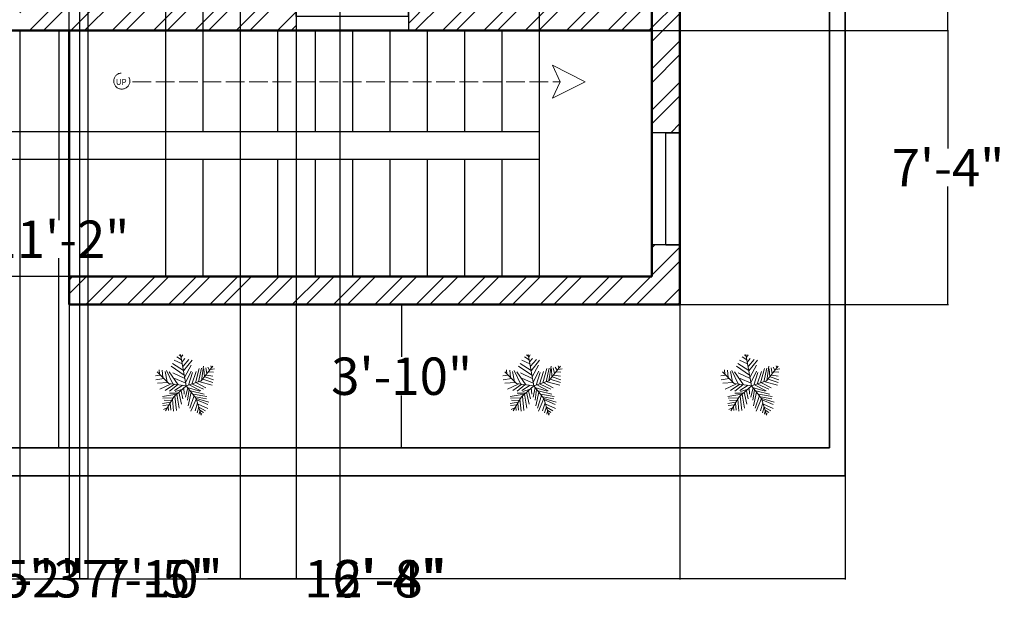
# Model space of a CAD drawing. Units: inches. Extents: x -40 to 578, y -482 to 237.
# Tile 2 of 7: x 219 to 535, y -482 to -295. Entities that reach past the tile are written whole.
import ezdxf

# ---------------------------------------------------------------- set-up
doc = ezdxf.new("R2010")
doc.units = ezdxf.units.IN
doc.header["$MEASUREMENT"] = 0
doc.linetypes.add('ACAD_ISO02W100', pattern=[15, 12, -3])
for name, color, linetype, lineweight in [('A-ANNO-DIMS', 2, 'Continuous', 18), ('A-ANNO-SYMB', 210, 'ACAD_ISO02W100', 18), ('A-FLOR-STRS', 210, 'Continuous', 25), ('A-WALL-PATT', 252, 'Continuous', 13), ('C-PROP', 3, 'Continuous', 35), ('L-PLNT', 94, 'Continuous', 13), ('WALLS', 3, 'Continuous', 50), ('WINDOWS', 241, 'Continuous', 25)]:
    doc.layers.add(name, color=color, linetype=linetype, lineweight=lineweight)
doc.styles.get("Standard").update_dxf_attribs({"font": 'arial.ttf'})
doc.dimstyles.get("Standard").update_dxf_attribs({"dimtxt": 12, "dimasz": 0.18, "dimexe": 0.18, "dimexo": 0.0625, "dimgap": 0.09, "dimtad": 0, "dimtih": 1, "dimtoh": 1, "dimdec": 0, "dimzin": 0, "dimdsep": 46, "dimlunit": 3, "dimtxsty": 'Standard', "dimcen": 0.09, "dimadec": 0, "dimazin": 0, "dimtfac": 1, "dimtdec": 0, "dimtofl": 0, "dimtmove": 0, "dimatfit": 3, "dimfxl": 1, "dimtolj": 1, "dimtzin": 0, "dimarcsym": 0})

# ---------------------------------------------------------------- blocks, each defined once
blk = doc.blocks.new('*U14')
for p, q in [((-258.7244, 1362.456), (-332.3336, 1421.4348)), ((0, 0), (-266.7, 1447.8)), ((-231.1146, 1315.2628), (-166.7002, 1421.4348)), ((-129.8956, 713.6638), (-626.7704, 1032.1544)), ((-185.1152, 1008.5578), (-553.1612, 1185.4942)), ((-221.9198, 1197.3052), (-433.5526, 1338.8594)), ((-194.31, 1102.9442), (-65.4812, 1256.284)), ((-148.3106, 914.1968), (118.5418, 1220.9018)), ((-129.8956, 701.8528), (265.7602, 1185.4942)), ((-74.7014, 418.7444), (219.7608, 961.39)), ((685.8, 228.6), (1219.2, 914.4)), ((689.0258, 230.0224), (790.2448, 914.1968)), ((1121.4862, 925.9824), (1149.0706, 831.6214)), ((-1206.4492, 501.3198), (-1418.082, 465.9376)), ((-800.1, 114.3), (-1333.5, 647.7)), ((-1234.059, 536.7274), (-1252.4486, 737.2604)), ((-1105.2302, 725.4494), (-1077.6458, 395.1732)), ((-976.4268, 666.4706), (-884.4026, 194.6402)), ((-902.8176, 713.6638), (-617.5756, 100.2538)), ((-369.1382, 53.086), (-783.1836, 642.874)), ((-93.091, 489.5342), (-700.3796, 902.3858)), ((-617.5756, 607.4918), (-74.7014, 347.98)), ((-28.6766, 171.0436), (228.9556, 678.2816)), ((100.1268, 41.275), (284.1498, 619.2774)), ((256.5654, 88.4682), (449.7832, 666.4706)), ((412.9786, 147.447), (587.8068, 796.2392)), ((560.197, 182.8292), (698.2206, 819.8358)), ((808.6344, 784.4282), (827.0494, 418.7444)), ((891.4384, 831.6214), (946.658, 572.1096)), ((919.0482, 501.3198), (1222.6798, 454.152)), ((983.4626, 867.0036), (1066.2666, 725.4494)), ((1029.462, 654.685), (1241.0948, 631.0884)), ((1112.2914, 760.8316), (1296.3144, 784.4282)), ((-1031.621, 347.98), (-1399.667, 277.1902)), ((-847.598, 159.2326), (-1326.0578, 135.636)), ((-718.7946, 88.4682), (-1215.644, -147.447)), ((-543.9664, 76.6572), (-967.2066, -206.4512)), ((0, 0), (-800.1, 114.3)), ((-405.9428, 53.086), (-764.794, -241.8334)), ((0, 0), (-571.5, -495.3)), ((-166.7002, 29.4894), (-543.9664, -206.4512)), ((-525.5514, 347.98), (-28.6766, 123.8504)), ((0, 0), (685.8, 228.6)), ((0, 0), (457.2, -571.5)), ((164.5412, 41.275), (661.416, -218.2368)), ((284.1498, 88.4682), (781.0246, -147.447)), ((458.978, 147.447), (891.4384, -88.4682)), ((615.4166, 194.6402), (1185.8752, 41.275)), ((753.4148, 312.5978), (1222.6798, 159.2326)), ((845.439, 418.7444), (1241.0948, 277.1902)), ((-442.7474, -383.3876), (-1086.8406, -477.7486)), ((-387.5278, -324.4088), (-764.794, -324.4088)), ((-166.7002, -147.447), (-507.1618, -253.619)), ((-433.5526, -383.3876), (-323.1134, -1020.3688)), ((-341.5284, -289.0012), (-221.9198, -831.6214)), ((-240.3094, -218.2368), (-157.5054, -595.7062)), ((-120.7008, -88.4682), (-93.091, -371.5766)), ((63.3222, -76.6826), (-37.8714, -513.1308)), ((44.9326, -64.897), (615.4166, -241.8334)), ((127.7366, -159.258), (54.1274, -654.685)), ((228.9556, -289.0012), (90.932, -914.1968)), ((357.759, -430.5554), (164.5412, -1020.3688)), ((192.151, -230.0224), (817.8292, -371.5766)), ((311.7596, -383.3876), (937.4378, -477.7486)), ((-718.7946, -737.2604), (-1086.8406, -796.2392)), ((-617.5756, -548.5384), (-1077.6458, -560.324)), ((-783.1836, -867.029), (-1077.6458, -902.4112)), ((-681.9646, -666.496), (-1022.4262, -654.685)), ((-571.5, -495.3), (-952.5, -1143)), ((-737.1842, -784.4536), (-709.5744, -1114.7298)), ((-635.9652, -607.5172), (-580.771, -1150.1374)), ((-525.5514, -465.963), (-451.9422, -1126.5408)), ((458.978, -572.1096), (210.5406, -1161.923)), ((514.1976, -772.6426), (403.7838, -1138.3264)), ((412.9786, -501.3452), (919.0482, -583.9206)), ((457.2, -571.5), (685.8, -1333.5)), ((468.1982, -572.1096), (1029.462, -737.2604)), ((486.5878, -642.8994), (983.4626, -843.4324)), ((541.8074, -831.6214), (992.6574, -1032.1544)), ((-875.2078, -1008.5832), (-1040.8412, -1079.3476)), ((-829.2084, -937.7934), (-810.7934, -1126.5408)), ((578.612, -961.39), (495.7826, -1232.7128)), ((578.612, -973.1756), (873.0488, -1138.3264)), ((624.6114, -1161.923), (587.8068, -1291.6916)), ((624.6114, -1102.9442), (781.0246, -1209.1162)), ((679.8056, -1268.095), (716.6102, -1291.6916))]:
    blk.add_line(p, q)
blk = doc.blocks.new('*D17')
at = {"layer": 'A-ANNO-DIMS', "color": 0, "lineweight": -2, "transparency": 16777216}
for p, q in [((229.86, -298.55), (231.51, -298.55)), ((231.33, -298.73), (231.33, -359.44)), ((231.33, -432.37), (231.33, -371.67)), ((229.86, -432.55), (231.51, -432.55))]:
    blk.add_line(p, q, dxfattribs=at)
at = {"layer": 'A-ANNO-DIMS', "color": 0, "transparency": 16777216}
for points in [[(231.3, -298.73), (231.36, -298.73), (231.33, -298.55)], [(231.3, -432.37), (231.36, -432.37), (231.33, -432.55)]]:
    blk.add_solid(points, dxfattribs=at)
at = {"layer": 'Defpoints', "color": 0, "transparency": 16777216}
for p in [(229.79, -298.55), (229.79, -432.55), (231.33, -432.55)]:
    blk.add_point(p, dxfattribs=at)
at = {"layer": 'A-ANNO-DIMS', "color": 0, "transparency": 16777216, "insert": (231.33, -365.55), "char_height": 12, "attachment_point": 5}
blk.add_mtext('\\A1;11\'-2"', dxfattribs=at)
blk = doc.blocks.new('*D18')
at = {"layer": 'A-ANNO-DIMS', "color": 0, "lineweight": -2, "transparency": 16777216}
for p, q in [((354.59, -386.55), (341.19, -386.55)), ((341.37, -386.73), (341.37, -403.33)), ((341.37, -432.37), (341.37, -415.77)), ((354.59, -432.55), (341.19, -432.55))]:
    blk.add_line(p, q, dxfattribs=at)
at = {"layer": 'A-ANNO-DIMS', "color": 0, "transparency": 16777216}
for points in [[(341.34, -386.73), (341.4, -386.73), (341.37, -386.55)], [(341.34, -432.37), (341.4, -432.37), (341.37, -432.55)]]:
    blk.add_solid(points, dxfattribs=at)
at = {"layer": 'Defpoints', "color": 0, "transparency": 16777216}
for p in [(354.65, -386.55), (341.37, -432.55), (354.65, -432.55)]:
    blk.add_point(p, dxfattribs=at)
at = {"layer": 'A-ANNO-DIMS', "color": 0, "transparency": 16777216, "insert": (341.37, -409.55), "char_height": 12, "attachment_point": 5}
blk.add_mtext('\\A1;3\'-10"', dxfattribs=at)
blk = doc.blocks.new('WIN-36IN')
for p, q in [((9, 36), (0, 36)), ((4.5, 0), (4.5, 36)), ((4.5, 36), (9, 36)), ((9, 0), (0, 0)), ((4.5, 0), (9, 0))]:
    blk.add_line(p, q)
blk = doc.blocks.new('*D38')
at = {"layer": 'A-ANNO-DIMS', "color": 0, "lineweight": -2, "transparency": 16777216}
for p, q in [((266.02, -266.84), (266.02, -263.91)), ((266.2, -264.09), (284.63, -264.09)), ((284.81, -266.84), (284.81, -263.91)), ((284.81, -264.09), (284.99, -264.09))]:
    blk.add_line(p, q, dxfattribs=at)
at = {"layer": 'A-ANNO-DIMS', "color": 0, "transparency": 16777216}
for points in [[(266.2, -264.06), (266.2, -264.12), (266.02, -264.09)], [(284.63, -264.06), (284.63, -264.12), (284.81, -264.09)]]:
    blk.add_solid(points, dxfattribs=at)
at = {"layer": 'Defpoints', "color": 0, "transparency": 16777216}
for p in [(284.81, -264.09), (266.02, -266.91), (284.81, -266.91)]:
    blk.add_point(p, dxfattribs=at)
at = {"layer": 'A-ANNO-DIMS', "color": 0, "transparency": 16777216, "insert": (370.24, -264.09), "char_height": 12, "attachment_point": 5}
blk.add_mtext('\\A1;END TABLE 1\'-7" TYP.', dxfattribs=at)
blk = doc.blocks.new('*D43')
at = {"layer": 'A-ANNO-DIMS', "color": 0, "lineweight": -2, "transparency": 16777216}
for p, q in [((29.74, -441.61), (29.74, -474.78)), ((483.74, -441.61), (483.74, -474.78)), ((29.92, -474.6), (231.38, -474.6)), ((483.56, -474.6), (282.1, -474.6))]:
    blk.add_line(p, q, dxfattribs=at)
at = {"layer": 'A-ANNO-DIMS', "color": 0, "transparency": 16777216}
for points in [[(29.92, -474.57), (29.92, -474.63), (29.74, -474.6)], [(483.56, -474.57), (483.56, -474.63), (483.74, -474.6)]]:
    blk.add_solid(points, dxfattribs=at)
at = {"layer": 'Defpoints', "color": 0, "transparency": 16777216}
for p in [(29.74, -441.55), (483.74, -441.55), (483.74, -474.6)]:
    blk.add_point(p, dxfattribs=at)
at = {"layer": 'A-ANNO-DIMS', "color": 0, "transparency": 16777216, "insert": (256.74, -474.6), "char_height": 12, "attachment_point": 5}
blk.add_mtext('\\A1;37\'-10"', dxfattribs=at)
blk = doc.blocks.new('*D47')
at = {"layer": 'A-ANNO-DIMS', "color": 0, "lineweight": -2, "transparency": 16777216}
for p, q in [((234.57, -386.61), (234.57, -474.78)), ((430.74, -386.61), (430.74, -474.78)), ((234.75, -474.6), (312.52, -474.6)), ((430.56, -474.6), (352.79, -474.6))]:
    blk.add_line(p, q, dxfattribs=at)
at = {"layer": 'A-ANNO-DIMS', "color": 0, "transparency": 16777216}
for points in [[(234.75, -474.57), (234.75, -474.63), (234.57, -474.6)], [(430.56, -474.57), (430.56, -474.63), (430.74, -474.6)]]:
    blk.add_solid(points, dxfattribs=at)
at = {"layer": 'Defpoints', "color": 0, "transparency": 16777216}
for p in [(234.57, -386.55), (430.74, -386.55), (430.74, -474.6)]:
    blk.add_point(p, dxfattribs=at)
at = {"layer": 'A-ANNO-DIMS', "color": 0, "transparency": 16777216, "insert": (332.66, -474.6), "char_height": 12, "attachment_point": 5}
blk.add_mtext('\\A1;16\'-4"', dxfattribs=at)
blk = doc.blocks.new('*D48')
at = {"layer": 'A-ANNO-DIMS', "color": 0, "lineweight": -2, "transparency": 16777216}
for p, q in [((430.800209, -298.552485), (516.967709, -298.552485)), ((516.787709, -298.732485), (516.787709, -336.462485)), ((516.787709, -386.372485), (516.787709, -348.642485)), ((430.800209, -386.552485), (516.967709, -386.552485))]:
    blk.add_line(p, q, dxfattribs=at)
at = {"layer": 'A-ANNO-DIMS', "color": 0, "transparency": 16777216}
for points in [[(516.757709, -298.732485), (516.817709, -298.732485), (516.787709, -298.552485)], [(516.757709, -386.372485), (516.817709, -386.372485), (516.787709, -386.552485)]]:
    blk.add_solid(points, dxfattribs=at)
at = {"layer": 'Defpoints', "color": 0, "transparency": 16777216}
for p in [(430.737709, -298.552485), (516.787709, -298.552485), (430.737709, -386.552485)]:
    blk.add_point(p, dxfattribs=at)
at = {"layer": 'A-ANNO-DIMS', "color": 0, "transparency": 16777216, "insert": (516.787709, -342.552485), "char_height": 12, "attachment_point": 5}
blk.add_mtext('\\A1;7\'-4"', dxfattribs=at)
blk = doc.blocks.new('*D49')
at = {"layer": 'A-ANNO-DIMS', "color": 0, "lineweight": -2, "transparency": 16777216}
for p, q in [((385.66, -377.49), (385.66, 219.12)), ((385.84, 218.94), (387.66, 218.94)), ((421.56, 218.94), (419.73, 218.94)), ((421.74, -377.49), (421.74, 219.12))]:
    blk.add_line(p, q, dxfattribs=at)
at = {"layer": 'A-ANNO-DIMS', "color": 0, "transparency": 16777216}
for points in [[(385.84, 218.97), (385.84, 218.91), (385.66, 218.94)], [(421.56, 218.97), (421.56, 218.91), (421.74, 218.94)]]:
    blk.add_solid(points, dxfattribs=at)
at = {"layer": 'Defpoints', "color": 0, "transparency": 16777216}
for p in [(421.74, 218.94), (385.66, -377.55), (421.74, -377.55)]:
    blk.add_point(p, dxfattribs=at)
at = {"layer": 'A-ANNO-DIMS', "color": 0, "transparency": 16777216, "insert": (403.7, 218.94), "char_height": 12, "attachment_point": 5}
blk.add_mtext('\\A1;3\'-0"', dxfattribs=at)
blk = doc.blocks.new('*D50')
at = {"layer": 'A-ANNO-DIMS', "color": 0, "lineweight": -2, "transparency": 16777216}
for p, q in [((265.66, -330.99), (265.66, 219.12)), ((265.84, 218.94), (277.48, 218.94)), ((277.66, -330.99), (277.66, 219.12)), ((277.66, 218.94), (277.84, 218.94))]:
    blk.add_line(p, q, dxfattribs=at)
at = {"layer": 'A-ANNO-DIMS', "color": 0, "transparency": 16777216}
for points in [[(265.84, 218.97), (265.84, 218.91), (265.66, 218.94)], [(277.48, 218.97), (277.48, 218.91), (277.66, 218.94)]]:
    blk.add_solid(points, dxfattribs=at)
at = {"layer": 'Defpoints', "color": 0, "transparency": 16777216}
for p in [(277.66, 218.94), (265.66, -331.05), (277.66, -331.05)]:
    blk.add_point(p, dxfattribs=at)
at = {"layer": 'A-ANNO-DIMS', "color": 0, "transparency": 16777216, "insert": (293.31, 218.94), "char_height": 12, "attachment_point": 5}
blk.add_mtext('\\A1;1\'-0"', dxfattribs=at)
blk = doc.blocks.new('*D51')
at = {"layer": 'A-ANNO-DIMS', "color": 0, "lineweight": -2, "transparency": 16777216}
for p, q in [((385.59, -298.55), (-3.49, -298.55)), ((-3.31, -298.73), (-3.31, -308.51)), ((-3.31, -330.87), (-3.31, -321.1)), ((385.59, -331.05), (-3.49, -331.05))]:
    blk.add_line(p, q, dxfattribs=at)
at = {"layer": 'A-ANNO-DIMS', "color": 0, "transparency": 16777216}
for points in [[(-3.34, -298.73), (-3.28, -298.73), (-3.31, -298.55)], [(-3.34, -330.87), (-3.28, -330.87), (-3.31, -331.05)]]:
    blk.add_solid(points, dxfattribs=at)
at = {"layer": 'Defpoints', "color": 0, "transparency": 16777216}
for p in [(385.66, -298.55), (-3.31, -331.05), (385.66, -331.05)]:
    blk.add_point(p, dxfattribs=at)
at = {"layer": 'A-ANNO-DIMS', "color": 0, "transparency": 16777216, "insert": (-3.31, -314.8), "char_height": 12, "attachment_point": 5}
blk.add_mtext('\\A1;2\'-8 1/2"', dxfattribs=at)
blk = doc.blocks.new('*D52')
at = {"layer": 'A-ANNO-DIMS', "color": 0, "lineweight": -2, "transparency": 16777216}
for p, q in [((234.57, -377.49), (234.57, 219.12)), ((234.75, 218.94), (265.48, 218.94)), ((265.66, -377.49), (265.66, 219.12)), ((265.66, 218.94), (265.84, 218.94))]:
    blk.add_line(p, q, dxfattribs=at)
at = {"layer": 'A-ANNO-DIMS', "color": 0, "transparency": 16777216}
for points in [[(234.75, 218.97), (234.75, 218.91), (234.57, 218.94)], [(265.48, 218.97), (265.48, 218.91), (265.66, 218.94)]]:
    blk.add_solid(points, dxfattribs=at)
at = {"layer": 'Defpoints', "color": 0, "transparency": 16777216}
for p in [(265.66, 218.94), (234.57, -377.55), (265.66, -377.55)]:
    blk.add_point(p, dxfattribs=at)
at = {"layer": 'A-ANNO-DIMS', "color": 0, "transparency": 16777216, "insert": (281.98, 218.94), "char_height": 12, "attachment_point": 5}
blk.add_mtext('\\A1;2\'-7"', dxfattribs=at)
blk = doc.blocks.new('*D53')
at = {"layer": 'A-ANNO-DIMS', "color": 0, "lineweight": -2, "transparency": 16777216}
for p, q in [((265.59, -339.94), (-3.49, -339.94)), ((-3.31, -340.12), (-3.31, -352.45)), ((-3.31, -377.37), (-3.31, -365.04)), ((265.59, -377.55), (-3.49, -377.55))]:
    blk.add_line(p, q, dxfattribs=at)
at = {"layer": 'A-ANNO-DIMS', "color": 0, "transparency": 16777216}
for points in [[(-3.34, -340.12), (-3.28, -340.12), (-3.31, -339.94)], [(-3.34, -377.37), (-3.28, -377.37), (-3.31, -377.55)]]:
    blk.add_solid(points, dxfattribs=at)
at = {"layer": 'Defpoints', "color": 0, "transparency": 16777216}
for p in [(265.66, -339.94), (-3.31, -377.55), (265.66, -377.55)]:
    blk.add_point(p, dxfattribs=at)
at = {"layer": 'A-ANNO-DIMS', "color": 0, "transparency": 16777216, "insert": (-3.31, -358.75), "char_height": 12, "attachment_point": 5}
blk.add_mtext('\\A1;3\'-1 1/2"', dxfattribs=at)
blk = doc.blocks.new('*D54')
at = {"layer": 'A-ANNO-DIMS', "color": 0, "lineweight": -2, "transparency": 16777216}
for p, q in [((202.4, 25.39), (202.4, -474.78)), ((240.62, 25.39), (240.62, -474.78)), ((202.58, -474.6), (205.48, -474.6)), ((240.44, -474.6), (237.55, -474.6))]:
    blk.add_line(p, q, dxfattribs=at)
at = {"layer": 'A-ANNO-DIMS', "color": 0, "transparency": 16777216}
for points in [[(202.58, -474.57), (202.58, -474.63), (202.4, -474.6)], [(240.44, -474.57), (240.44, -474.63), (240.62, -474.6)]]:
    blk.add_solid(points, dxfattribs=at)
at = {"layer": 'Defpoints', "color": 0, "transparency": 16777216}
for p in [(202.4, 25.45), (240.62, 25.45), (240.62, -474.6)]:
    blk.add_point(p, dxfattribs=at)
at = {"layer": 'A-ANNO-DIMS', "color": 0, "transparency": 16777216, "insert": (221.51, -474.6), "char_height": 12, "attachment_point": 5}
blk.add_mtext('\\A1;3\'-2"', dxfattribs=at)
blk = doc.blocks.new('*D69')
at = {"layer": 'A-ANNO-DIMS', "color": 0, "lineweight": -2, "transparency": 16777216}
for p, q in [((321.5, -125.98), (321.5, -474.78)), ((289.56, -128.61), (289.56, -474.78)), ((289.74, -474.6), (321.32, -474.6)), ((321.5, -474.6), (321.68, -474.6))]:
    blk.add_line(p, q, dxfattribs=at)
at = {"layer": 'A-ANNO-DIMS', "color": 0, "transparency": 16777216}
for points in [[(289.74, -474.57), (289.74, -474.63), (289.56, -474.6)], [(321.32, -474.57), (321.32, -474.63), (321.5, -474.6)]]:
    blk.add_solid(points, dxfattribs=at)
at = {"layer": 'Defpoints', "color": 0, "transparency": 16777216}
for p in [(321.5, -125.92), (289.56, -128.55), (321.5, -474.6)]:
    blk.add_point(p, dxfattribs=at)
at = {"layer": 'A-ANNO-DIMS', "color": 0, "transparency": 16777216, "insert": (337.82, -474.6), "char_height": 12, "attachment_point": 5}
blk.add_mtext('\\A1;2\'-8"', dxfattribs=at)
blk = doc.blocks.new('*D71')
at = {"layer": 'A-ANNO-DIMS', "color": 0, "lineweight": -2, "transparency": 16777216}
for p, q in [((184.88, -63.19), (184.88, -474.78)), ((237.97, -63.19), (237.97, -474.78)), ((185.06, -474.6), (195.15, -474.6)), ((237.79, -474.6), (227.71, -474.6))]:
    blk.add_line(p, q, dxfattribs=at)
at = {"layer": 'A-ANNO-DIMS', "color": 0, "transparency": 16777216}
for points in [[(185.06, -474.57), (185.06, -474.63), (184.88, -474.6)], [(237.79, -474.57), (237.79, -474.63), (237.97, -474.6)]]:
    blk.add_solid(points, dxfattribs=at)
at = {"layer": 'Defpoints', "color": 0, "transparency": 16777216}
for p in [(184.88, -63.12), (237.97, -63.12), (237.97, -474.6)]:
    blk.add_point(p, dxfattribs=at)
at = {"layer": 'A-ANNO-DIMS', "color": 0, "transparency": 16777216, "insert": (211.43, -474.6), "char_height": 12, "attachment_point": 5}
blk.add_mtext('\\A1;4\'-5"', dxfattribs=at)
blk = doc.blocks.new('*D78')
at = {"layer": 'A-ANNO-DIMS', "color": 0, "lineweight": -2, "transparency": 16777216}
for p, q in [((430.8, -233.77), (516.97, -233.77)), ((516.79, -233.95), (516.79, -259.97)), ((516.79, -298.37), (516.79, -272.35)), ((421.8, -298.55), (516.97, -298.55))]:
    blk.add_line(p, q, dxfattribs=at)
at = {"layer": 'A-ANNO-DIMS', "color": 0, "transparency": 16777216}
for points in [[(516.76, -233.95), (516.82, -233.95), (516.79, -233.77)], [(516.76, -298.37), (516.82, -298.37), (516.79, -298.55)]]:
    blk.add_solid(points, dxfattribs=at)
at = {"layer": 'Defpoints', "color": 0, "transparency": 16777216}
for p in [(430.74, -233.77), (421.74, -298.55), (516.79, -298.55)]:
    blk.add_point(p, dxfattribs=at)
at = {"layer": 'A-ANNO-DIMS', "color": 0, "transparency": 16777216, "insert": (516.79, -266.16), "char_height": 12, "attachment_point": 5}
blk.add_mtext('\\A1;5\'-5"', dxfattribs=at)
blk = doc.blocks.new('*D80')
at = {"layer": 'A-ANNO-DIMS', "color": 0, "lineweight": -2, "transparency": 16777216}
for p, q in [((218.74, -298.61), (218.74, -474.78)), ((307.53, -298.61), (307.53, -474.78)), ((218.92, -474.6), (247.14, -474.6)), ((307.35, -474.6), (279.13, -474.6))]:
    blk.add_line(p, q, dxfattribs=at)
at = {"layer": 'A-ANNO-DIMS', "color": 0, "transparency": 16777216}
for points in [[(218.92, -474.57), (218.92, -474.63), (218.74, -474.6)], [(307.35, -474.57), (307.35, -474.63), (307.53, -474.6)]]:
    blk.add_solid(points, dxfattribs=at)
at = {"layer": 'Defpoints', "color": 0, "transparency": 16777216}
for p in [(218.74, -298.55), (307.53, -298.55), (307.53, -474.6)]:
    blk.add_point(p, dxfattribs=at)
at = {"layer": 'A-ANNO-DIMS', "color": 0, "transparency": 16777216, "insert": (263.14, -474.6), "char_height": 12, "attachment_point": 5}
blk.add_mtext('\\A1;7\'-5"', dxfattribs=at)

msp = doc.modelspace()

# ---------------------------------------------------------------- hatches: boundary and pattern name
at = {"layer": 'A-WALL-PATT'}
h = msp.add_hatch(dxfattribs=at)
h.set_pattern_fill('ANSI32', color=256, scale=25)
h.set_pattern_definition([(45, (-1993.713, -1175.095), (-6.629126, 6.629126), []), (45, (-1989.294, -1175.095), (-6.629126, 6.629126), [])])
h.paths.add_polyline_path([(248.74, 172.45), (71.74, 172.45), (71.74, 114.63), (80.74, 114.63), (80.74, 163.45), (248.74, 163.45)])
h.paths.add_polyline_path([(253.74, 172.45), (248.74, 172.45), (248.74, 163.45), (253.74, 163.45)])
h.paths.add_polyline_path([(253.74, 163.45), (248.74, 163.45), (248.74, 25.45), (240.62, 25.45), (240.62, 20.45), (263.71, 20.45), (263.71, 25.45), (253.74, 25.45)])
h.paths.add_polyline_path([(483.74, 172.45), (253.74, 172.45), (253.74, 163.45), (426.74, 163.45), (474.74, 163.45), (474.74, 79.45), (465.23, 79.45), (465.23, 77.2), (441.23, 77.2), (441.23, 74.45), (483.74, 74.45)])
h.paths.add_polyline_path([(80.74, 78.63), (71.74, 78.63), (71.74, 3.32), (80.74, 3.32), (80.74, 20.45), (134.6, 20.45), (134.6, 25.45), (80.74, 25.45)])
h.paths.add_polyline_path([(202.4, 25.45), (158.53, 25.45), (158.53, 20.45), (202.4, 20.45)])
h.paths.add_polyline_path([(169.74, 20.45), (164.74, 20.45), (164.74, -39.55), (80.74, -39.55), (80.74, -20.68), (71.74, -20.68), (71.74, -61.38), (80.74, -61.38), (80.74, -44.55), (164.74, -44.55), (164.74, -104.55), (169.74, -104.55), (169.74, -44.55)])
h.paths.add_polyline_path([(135.96, -104.55), (80.74, -104.55), (80.74, -85.38), (71.74, -85.38), (71.74, -155.89), (80.74, -155.89), (80.74, -109.55), (135.96, -109.55)])
h.paths.add_polyline_path([(218.74, -104.55), (159.9, -104.55), (159.9, -109.55), (218.74, -109.55)])
h.paths.add_polyline_path([(223.74, -104.55), (218.74, -104.55), (218.74, -109.55), (223.74, -109.55)])
h.paths.add_polyline_path([(223.74, -109.55), (218.74, -109.55), (218.74, -114.58), (223.74, -114.58)])
h.paths.add_polyline_path([(430.74, -85.66), (421.74, -85.66), (421.74, -128.55), (223.74, -128.55), (223.74, -133.55), (421.74, -133.55), (421.74, -197.77), (430.74, -197.77)])
h.paths.add_polyline_path([(223.74, -152.8), (218.74, -152.8), (218.74, -229.55), (151.59, -229.55), (151.59, -238.55), (223.74, -238.55), (223.74, -229.55)])
h.paths.add_polyline_path([(115.59, -229.55), (98.23, -229.55), (80.74, -229.55), (80.74, -212.75), (80.74, -191.89), (71.74, -191.89), (71.74, -238.55), (115.59, -238.55)])
h.paths.add_polyline_path([(307.53, -289.55), (223.74, -289.55), (223.74, -283.47), (218.74, -283.47), (218.74, -298.55), (307.53, -298.55)])
h.paths.add_polyline_path([(421.74, -289.55), (343.53, -289.55), (343.53, -298.55), (421.74, -298.55)])
h.paths.add_polyline_path([(430.74, -367.34), (421.74, -367.34), (421.74, -377.55), (234.57, -377.55), (234.57, -386.55), (430.74, -386.55)])
h.paths.add_polyline_path([(430.74, -298.55), (430.74, -233.77), (421.74, -233.77), (421.74, -289.55), (421.74, -298.55), (421.74, -331.34), (430.74, -331.34)])
h.paths.add_polyline_path([(430.74, -11.67), (427.15, -11.67, -0.057068), (421.74, -11.05), (421.74, -49.66), (430.74, -49.66)])
h.paths.add_polyline_path([(430.74, 31.9), (421.74, 31.9), (421.74, 25.45), (301.93, 25.45), (301.93, 20.45), (421.74, 20.45), (421.74, 12.26), (430.74, 12.26)])
h.paths.add_polyline_path([(426.74, 134.23, -0.014739), (425.33, 134.19), (421.74, 134.19), (421.74, 74.45), (441.23, 74.45), (441.23, 77.2), (441.23, 79.45), (426.74, 79.45)], flags=17)
h.paths.add_polyline_path([(430.74, 74.45), (421.74, 74.45), (421.74, 67.9), (430.74, 67.9)])

# ---------------------------------------------------------------- linework, layer by layer
at = {"layer": 'A-ANNO-SYMB'}
for p, q in [((392.27, -314.97), (389.86, -309.7)), ((389.86, -309.7), (400.34, -314.97)), ((392.27, -314.97), (389.86, -320.24)), ((389.86, -320.24), (400.34, -314.97))]:
    msp.add_line(p, q, dxfattribs=at)
at = {"layer": 'A-ANNO-SYMB', "ltscale": 0.5}
msp.add_line((254.95, -314.97), (392.27, -314.97), dxfattribs=at)
at = {"layer": 'A-ANNO-SYMB'}
msp.add_circle((251.52, -314.77), 2.59, dxfattribs=at)
at = {"layer": 'A-FLOR-STRS'}
for p, q in [((265.66, -333.55), (265.66, -298.55)), ((277.66, -331.05), (277.66, -298.55)), ((289.66, -331.05), (289.66, -298.55)), ((301.66, -331.05), (301.66, -298.55)), ((313.66, -331.05), (313.66, -298.55)), ((325.66, -331.05), (325.66, -298.55)), ((337.66, -331.05), (337.66, -298.55)), ((349.66, -331.05), (349.66, -298.55)), ((361.66, -331.05), (361.66, -298.55)), ((373.66, -331.05), (373.66, -298.55)), ((385.66, -333.55), (385.66, -298.55)), ((385.66, -331.05), (265.66, -331.05)), ((265.66, -377.55), (265.66, -333.55)), ((385.66, -377.55), (385.66, -333.55)), ((385.66, -339.94), (265.66, -339.94)), ((277.66, -377.55), (277.66, -339.94)), ((289.66, -377.55), (289.66, -339.94)), ((301.66, -377.55), (301.66, -339.94)), ((313.66, -377.55), (313.66, -339.94)), ((325.66, -377.55), (325.66, -339.94)), ((337.66, -377.55), (337.66, -339.94)), ((349.66, -377.55), (349.66, -339.94)), ((361.66, -377.55), (361.66, -339.94)), ((373.66, -377.55), (373.66, -339.94))]:
    msp.add_line(p, q, dxfattribs=at)
at = {"layer": 'C-PROP'}
for p, q in [((478.74, 74.45), (478.74, -432.55)), ((483.74, 74.45), (483.74, -441.55)), ((478.74, -432.55), (34.74, -432.55)), ((483.74, -441.55), (29.74, -441.55))]:
    msp.add_line(p, q, dxfattribs=at)
at = {"layer": 'WALLS'}
for p, q in [((430.74, 74.45), (430.74, -298.55)), ((421.74, -289.55), (421.74, -377.55)), ((213.16, -298.55), (421.74, -298.55)), ((234.57, -298.55), (234.57, -386.55)), ((430.74, -298.55), (430.74, -386.55)), ((421.74, -377.55), (234.57, -377.55)), ((430.74, -386.55), (234.57, -386.55))]:
    msp.add_line(p, q, dxfattribs=at)

# ---------------------------------------------------------------- block references
at = {"layer": 'L-PLNT', "xscale": 0.0070029080995801, "yscale": 0.0070029080995801, "zscale": 0.0070029080995801}
for p in [(272.24, -412.68), (383.82, -412.68), (453.75, -412.68)]:
    msp.add_blockref('*U14', p, dxfattribs=at)
at = {"layer": 'WINDOWS', "rotation": 90.0000000000001}
msp.add_blockref('WIN-36IN', (343.53, -298.55), dxfattribs=at)
at = {"layer": 'WINDOWS'}
msp.add_blockref('WIN-36IN', (421.74, -367.34), dxfattribs=at)

# ---------------------------------------------------------------- texts
at = {"layer": 'A-ANNO-SYMB'}
msp.add_text('UP', height=1.866, dxfattribs=at).set_placement((249.61, -316))

# ---------------------------------------------------------------- dimensions: what is measured, and where the dimension line sits
at = {"layer": 'A-ANNO-DIMS'}
for base, p1, p2, picture, middle in [((265.66, 218.94), (234.57, -377.55), (265.66, -377.55), '*D52', (281.98, 218.94)), ((277.66, 218.94), (265.66, -331.05), (277.66, -331.05), '*D50', (293.31, 218.94)), ((421.74, 218.94), (385.66, -377.55), (421.74, -377.55), '*D49', (403.7, 218.94)), ((240.62, -474.6), (202.4, 25.45), (240.62, 25.45), '*D54', (221.51, -474.6)), ((237.97, -474.6), (184.88, -63.12), (237.97, -63.12), '*D71', (211.43, -474.6)), ((321.5, -474.6), (289.56, -128.55), (321.5, -125.92), '*D69', (337.82, -474.6)), ((307.53, -474.6), (218.74, -298.55), (307.53, -298.55), '*D80', (263.14, -474.6)), ((430.74, -474.6), (234.57, -386.55), (430.74, -386.55), '*D47', (332.66, -474.6)), ((483.74, -474.6), (29.74, -441.55), (483.74, -441.55), '*D43', (256.74, -474.6))]:
    dim = msp.add_linear_dim(base=base, p1=p1, p2=p2, dimstyle='Standard', override={"dimdec": 1, "dimlfac": 1, "dimrnd": 0, "dimzin": 1, "dimdsep": 46, "dimlunit": 4, "dimfrac": 2}, dxfattribs=at)
    dim.commit()
    dim.dimension.update_dxf_attribs({"geometry": picture, "text_midpoint": middle})
dim = msp.add_linear_dim(base=(284.81, -264.09), p1=(266.02, -266.91), p2=(284.81, -266.91), text='END TABLE <> TYP.', dimstyle='Standard', override={"dimdec": 1, "dimlfac": 1, "dimrnd": 0, "dimzin": 1, "dimdsep": 46, "dimlunit": 4, "dimfrac": 2}, dxfattribs=at)
dim.commit()
dim.dimension.update_dxf_attribs({"geometry": '*D38', "text_midpoint": (370.24, -264.09)})
for base, p1, p2, override, picture, middle in [((516.79, -298.55), (430.74, -233.77), (421.74, -298.55), {"dimdec": 1, "dimlfac": 1, "dimrnd": 0, "dimzin": 1, "dimdsep": 46, "dimlunit": 4, "dimfrac": 2}, '*D78', (516.79, -266.16)), ((-3.31, -331.05), (385.66, -298.55), (385.66, -331.05), {"dimdec": 1, "dimlfac": 1, "dimrnd": 0, "dimzin": 1, "dimdsep": 46, "dimlunit": 4, "dimfrac": 2}, '*D51', (-3.31, -314.8)), ((231.33, -432.55), (229.79, -298.55), (229.79, -432.55), {"dimclrd": 0, "dimclre": 0, "dimclrt": 0}, '*D17', (231.33, -365.55)), ((516.79, -298.55), (430.74, -386.55), (430.74, -298.55), {"dimdec": 1, "dimlfac": 1, "dimrnd": 0, "dimzin": 1, "dimdsep": 46, "dimlunit": 4, "dimfrac": 2}, '*D48', (516.79, -342.55)), ((-3.31, -377.55), (265.66, -339.94), (265.66, -377.55), {"dimdec": 1, "dimlfac": 1, "dimrnd": 0, "dimzin": 1, "dimdsep": 46, "dimlunit": 4, "dimfrac": 2}, '*D53', (-3.31, -358.75)), ((341.37, -432.55), (354.65, -386.55), (354.65, -432.55), {"dimclrd": 0, "dimclre": 0, "dimclrt": 0}, '*D18', (341.37, -409.55))]:
    dim = msp.add_linear_dim(base=base, p1=p1, p2=p2, angle=90, dimstyle='Standard', override=override, dxfattribs=at)
    dim.commit()
    dim.dimension.update_dxf_attribs({"geometry": picture, "text_midpoint": middle})

doc.saveas('drawing.dxf')
